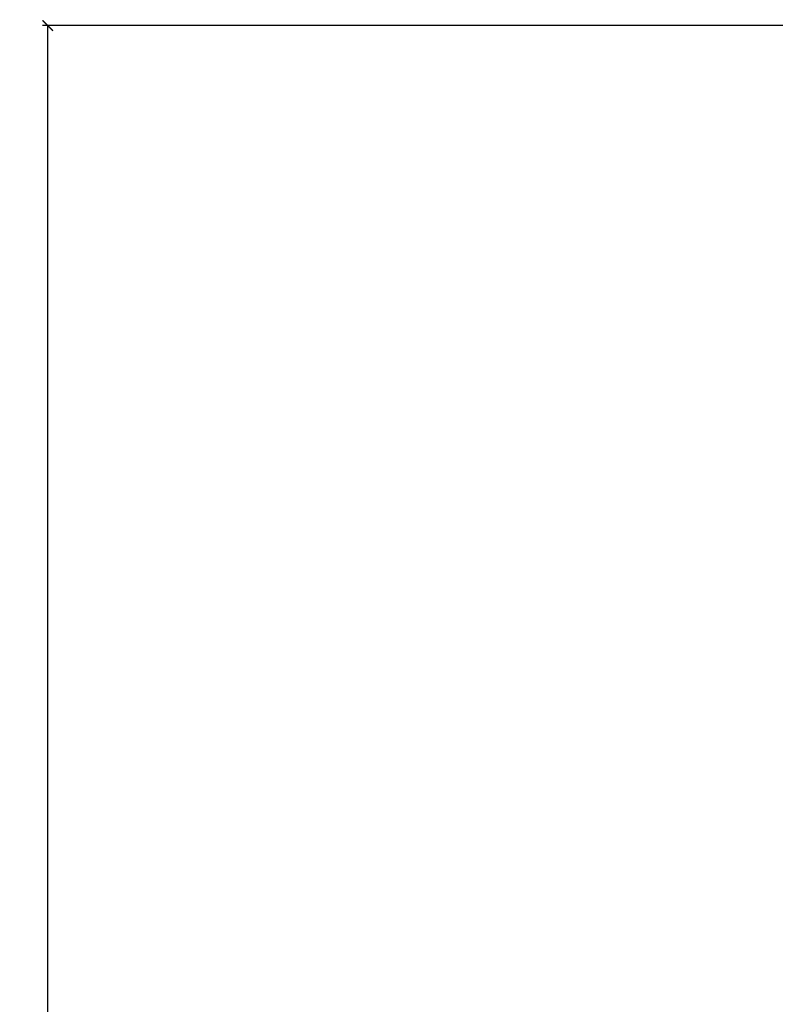
# Model space of a CAD drawing. Units: inches. Extents: x 3283068 to 3284536, y 3240756 to 3241803.
# Tile 7 of 19: x 3283068 to 3283246, y 3241501 to 3241732. Entities that reach past the tile are written whole.
import ezdxf

# ---------------------------------------------------------------- set-up
doc = ezdxf.new("R2010")
doc.units = ezdxf.units.IN
doc.layers.add('A-ANNO-DIMS', color=2, linetype='Continuous', lineweight=18)
doc.styles.get("Standard").update_dxf_attribs({"font": 'arial.ttf'})
doc.dimstyles.new('ISO-25', dxfattribs={"dimtxt": 5, "dimasz": 2.5, "dimexe": 1.25, "dimexo": 0.625, "dimtad": 1, "dimlunit": 4, "dimtxsty": 'Standard', "dimblk": 'ARCHTICK', "dimcen": 2.5, "dimadec": 0, "dimazin": 0, "dimtfac": 1, "dimtmove": 0, "dimatfit": 3, "dimfxl": 1, "dimarcsym": 0})

# ---------------------------------------------------------------- blocks, each defined once
blk = doc.blocks.new('_ArchTick')
at = {"color": 0, "linetype": 'ByBlock', "const_width": 0.15}
blk.add_lwpolyline([(-0.5, -0.5), (0.5, 0.5)], dxfattribs=at)
blk = doc.blocks.new('*D61')
at = {"layer": 'A-ANNO-DIMS', "color": 0, "lineweight": -2, "transparency": 16777216}
for p, q in [((3283247.46, 3241730.6), (3283073.57, 3241730.6)), ((3283074.82, 3241082.6), (3283074.82, 3241730.6)), ((3283247.46, 3241082.6), (3283073.57, 3241082.6))]:
    blk.add_line(p, q, dxfattribs=at)
at = {"layer": 'Defpoints', "color": 0, "transparency": 16777216}
for p in [(3283074.82, 3241730.6), (3283248.09, 3241730.6), (3283248.09, 3241082.6)]:
    blk.add_point(p, dxfattribs=at)
at = {"layer": 'A-ANNO-DIMS', "color": 0, "lineweight": -2, "transparency": 16777216, "xscale": 2.5, "yscale": 2.5, "zscale": 2.5}
for p, rotation in [((3283074.82, 3241730.6), 90), ((3283074.82, 3241082.6), 270)]:
    blk.add_blockref('_ArchTick', p, dxfattribs=dict(at, rotation=rotation))
at = {"layer": 'A-ANNO-DIMS', "color": 0, "transparency": 16777216, "insert": (3283071.64, 3241406.6), "char_height": 5, "attachment_point": 5, "rotation": 90}
blk.add_mtext('54\'-0"', dxfattribs=at)

msp = doc.modelspace()

# ---------------------------------------------------------------- dimensions: what is measured, and where the dimension line sits
at = {"layer": 'A-ANNO-DIMS'}
dim = msp.add_linear_dim(base=(3283074.817, 3241730.602), p1=(3283248.089, 3241082.602), p2=(3283248.089, 3241730.602), angle=90, dimstyle='ISO-25', override={"dimdec": 1, "dimlfac": 1, "dimrnd": 0, "dimzin": 1, "dimdsep": 46, "dimlunit": 4, "dimfrac": 2}, dxfattribs=at)
dim.commit()
dim.dimension.update_dxf_attribs({"geometry": '*D61', "text_midpoint": (3283071.639, 3241406.602)})

doc.saveas('drawing.dxf')
